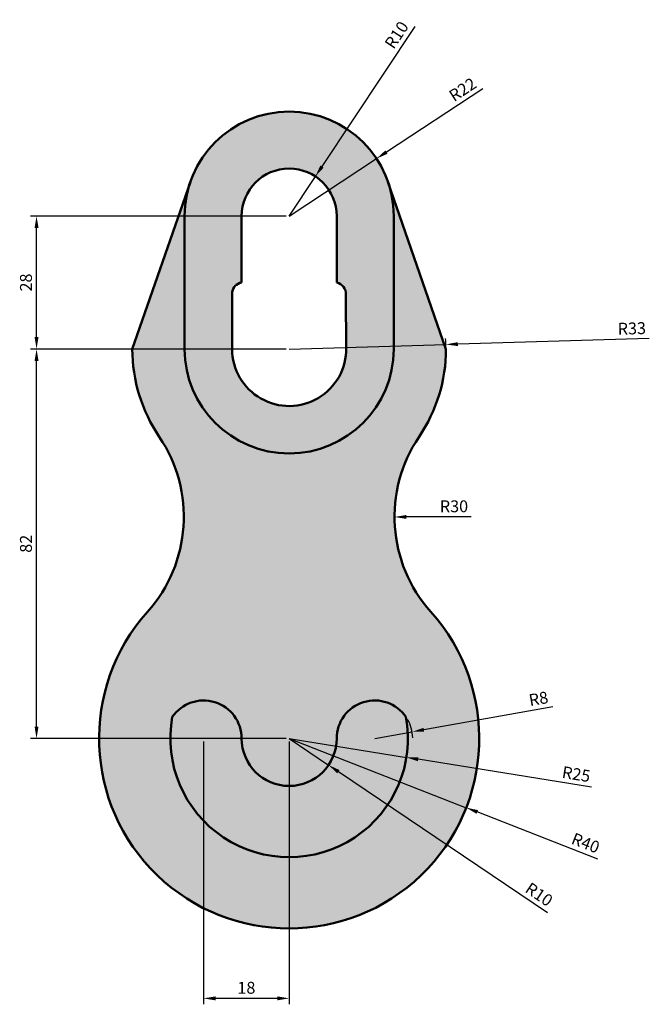
# Model space of a CAD drawing. Units: millimetres. Extents: x 3096 to 3229, y 1131 to 1338.
import ezdxf

# ---------------------------------------------------------------- set-up
doc = ezdxf.new("R2010")
doc.units = ezdxf.units.MM
for name, color, linetype, lineweight in [('M-DIMS', 2, 'Continuous', 25), ('M-HATC', 6, 'Continuous', 18), ('M-OUTL', 7, 'Continuous', 50)]:
    doc.layers.add(name, color=color, linetype=linetype, lineweight=lineweight)
doc.styles.get("Standard").update_dxf_attribs({"font": 'arial.ttf'})
doc.dimstyles.new('ISO-25', dxfattribs={"dimtxt": 2.5, "dimasz": 2.5, "dimexe": 1.25, "dimexo": 0.625, "dimtad": 1, "dimtxsty": 'Standard', "dimcen": 2.5, "dimadec": 0, "dimazin": 0, "dimtfac": 1, "dimtmove": 0, "dimatfit": 3, "dimfxl": 1, "dimarcsym": 0})

# ---------------------------------------------------------------- blocks, each defined once
blk = doc.blocks.new('*D1')
at = {"layer": 'Defpoints', "color": 0, "transparency": 16777216}
for p in [(3171.52, 1308.89), (3153.14, 1296.8)]:
    blk.add_point(p, dxfattribs=at)
at = {"layer": 'M-DIMS', "color": 0, "lineweight": -2, "transparency": 16777216}
for p, q in [((3193.86, 1323.58), (3173.61, 1310.26)), ((3153.14, 1296.8), (3171.52, 1308.89))]:
    blk.add_line(p, q, dxfattribs=at)
at = {"layer": 'M-DIMS', "color": 0, "transparency": 16777216}
blk.add_solid([(3173.38, 1310.61), (3173.84, 1309.91), (3171.52, 1308.89)], dxfattribs=at)
at = {"layer": 'M-DIMS', "color": 0, "transparency": 16777216, "insert": (3189.82, 1323.17), "char_height": 2.5, "attachment_point": 5, "rotation": 33.3268}
blk.add_mtext('R22', dxfattribs=at)
blk = doc.blocks.new('*D2')
at = {"layer": 'Defpoints', "color": 0, "transparency": 16777216}
for p in [(3158.66, 1305.14), (3153.14, 1296.8)]:
    blk.add_point(p, dxfattribs=at)
at = {"layer": 'M-DIMS', "color": 0, "lineweight": -2, "transparency": 16777216}
for p, q in [((3179.59, 1336.71), (3160.04, 1307.22)), ((3153.14, 1296.8), (3158.66, 1305.14))]:
    blk.add_line(p, q, dxfattribs=at)
at = {"layer": 'M-DIMS', "color": 0, "transparency": 16777216}
blk.add_solid([(3159.7, 1307.45), (3160.39, 1306.99), (3158.66, 1305.14)], dxfattribs=at)
at = {"layer": 'M-DIMS', "color": 0, "transparency": 16777216, "insert": (3176.01, 1334.75), "char_height": 2.5, "attachment_point": 5, "rotation": 56.4616}
blk.add_mtext('R10', dxfattribs=at)
blk = doc.blocks.new('*D3')
at = {"layer": 'Defpoints', "color": 0, "transparency": 16777216}
for p in [(3153.14, 1268.8), (3186.12, 1269.76)]:
    blk.add_point(p, dxfattribs=at)
at = {"layer": 'M-DIMS', "color": 0, "lineweight": -2, "transparency": 16777216}
for p, q in [((3228.92, 1271.01), (3188.62, 1269.84)), ((3153.14, 1268.8), (3186.12, 1269.76))]:
    blk.add_line(p, q, dxfattribs=at)
blk.add_arc((3153.14, 1268.8), 33, 1.0851, 3.843, dxfattribs=at)
at = {"layer": 'M-DIMS', "color": 0, "transparency": 16777216}
blk.add_solid([(3188.61, 1270.25), (3188.64, 1269.42), (3186.12, 1269.76)], dxfattribs=at)
at = {"layer": 'M-DIMS', "color": 0, "transparency": 16777216, "insert": (3225.25, 1272.81), "char_height": 2.5, "attachment_point": 5, "rotation": 1.6728}
blk.add_mtext('R33', dxfattribs=at)
blk = doc.blocks.new('*D4')
at = {"layer": 'Defpoints', "color": 0, "transparency": 16777216}
for p in [(3175.3, 1233.44), (3205.3, 1233.48)]:
    blk.add_point(p, dxfattribs=at)
at = {"layer": 'M-DIMS', "color": 0, "lineweight": -2, "transparency": 16777216}
blk.add_line((3191.43, 1233.46), (3177.8, 1233.45), dxfattribs=at)
at = {"layer": 'M-DIMS', "color": 0, "transparency": 16777216}
blk.add_solid([(3177.8, 1233.86), (3177.8, 1233.03), (3175.3, 1233.44)], dxfattribs=at)
at = {"layer": 'M-DIMS', "color": 0, "transparency": 16777216, "insert": (3187.82, 1235.36), "char_height": 2.5, "attachment_point": 5, "rotation": 0.0644}
blk.add_mtext('R30', dxfattribs=at)
blk = doc.blocks.new('*D5')
at = {"layer": 'Defpoints', "color": 0, "transparency": 16777216}
for p in [(3179.02, 1188.2), (3171.14, 1186.8)]:
    blk.add_point(p, dxfattribs=at)
at = {"layer": 'M-DIMS', "color": 0, "lineweight": -2, "transparency": 16777216}
for p, q in [((3208.6, 1193.44), (3181.48, 1188.63)), ((3171.14, 1186.8), (3179.02, 1188.2))]:
    blk.add_line(p, q, dxfattribs=at)
blk.add_arc((3171.14, 1186.8), 8, 1.1021, 30.1459, dxfattribs=at)
at = {"layer": 'M-DIMS', "color": 0, "transparency": 16777216}
blk.add_solid([(3181.4, 1189.04), (3181.55, 1188.22), (3179.02, 1188.2)], dxfattribs=at)
at = {"layer": 'M-DIMS', "color": 0, "transparency": 16777216, "insert": (3205.66, 1194.85), "char_height": 2.5, "attachment_point": 5, "rotation": 10.0546}
blk.add_mtext('R8', dxfattribs=at)
blk = doc.blocks.new('*D6')
at = {"layer": 'Defpoints', "color": 0, "transparency": 16777216}
for p in [(3153.14, 1186.8), (3177.82, 1182.81)]:
    blk.add_point(p, dxfattribs=at)
at = {"layer": 'M-DIMS', "color": 0, "lineweight": -2, "transparency": 16777216}
for p, q in [((3153.14, 1186.8), (3177.82, 1182.81)), ((3216.76, 1176.52), (3180.29, 1182.41))]:
    blk.add_line(p, q, dxfattribs=at)
at = {"layer": 'M-DIMS', "color": 0, "transparency": 16777216}
blk.add_solid([(3180.35, 1182.82), (3180.22, 1182), (3177.82, 1182.81)], dxfattribs=at)
at = {"layer": 'M-DIMS', "color": 0, "transparency": 16777216, "insert": (3213.49, 1178.97), "char_height": 2.5, "attachment_point": 5, "rotation": 350.8174}
blk.add_mtext('R25', dxfattribs=at)
blk = doc.blocks.new('*D7')
at = {"layer": 'Defpoints', "color": 0, "transparency": 16777216}
for p in [(3153.14, 1186.8), (3161.43, 1181.2)]:
    blk.add_point(p, dxfattribs=at)
at = {"layer": 'M-DIMS', "color": 0, "lineweight": -2, "transparency": 16777216}
for p, q in [((3153.14, 1186.8), (3161.43, 1181.2)), ((3207.47, 1150.11), (3163.5, 1179.8))]:
    blk.add_line(p, q, dxfattribs=at)
at = {"layer": 'M-DIMS', "color": 0, "transparency": 16777216}
blk.add_solid([(3163.73, 1180.15), (3163.26, 1179.46), (3161.43, 1181.2)], dxfattribs=at)
at = {"layer": 'M-DIMS', "color": 0, "transparency": 16777216, "insert": (3205.55, 1153.7), "char_height": 2.5, "attachment_point": 5, "rotation": 325.9669}
blk.add_mtext('R10', dxfattribs=at)
blk = doc.blocks.new('*D8')
at = {"layer": 'Defpoints', "color": 0, "transparency": 16777216}
for p in [(3153.14, 1186.8), (3190.39, 1172.23)]:
    blk.add_point(p, dxfattribs=at)
at = {"layer": 'M-DIMS', "color": 0, "lineweight": -2, "transparency": 16777216}
for p, q in [((3153.14, 1186.8), (3190.39, 1172.23)), ((3218.06, 1161.4), (3192.72, 1171.32))]:
    blk.add_line(p, q, dxfattribs=at)
at = {"layer": 'M-DIMS', "color": 0, "transparency": 16777216}
blk.add_solid([(3192.87, 1171.71), (3192.57, 1170.93), (3190.39, 1172.23)], dxfattribs=at)
at = {"layer": 'M-DIMS', "color": 0, "transparency": 16777216, "insert": (3215.4, 1164.49), "char_height": 2.5, "attachment_point": 5, "rotation": 338.6363}
blk.add_mtext('R40', dxfattribs=at)
blk = doc.blocks.new('*D9')
at = {"layer": 'Defpoints', "color": 0, "transparency": 16777216}
for p in [(3099.98, 1268.8), (3153.14, 1268.8), (3153.14, 1186.8)]:
    blk.add_point(p, dxfattribs=at)
at = {"layer": 'M-DIMS', "color": 0, "lineweight": -2, "transparency": 16777216}
for p, q in [((3152.51, 1268.8), (3098.73, 1268.8)), ((3099.98, 1189.3), (3099.98, 1266.3)), ((3152.51, 1186.8), (3098.73, 1186.8))]:
    blk.add_line(p, q, dxfattribs=at)
at = {"layer": 'M-DIMS', "color": 0, "transparency": 16777216}
for points in [[(3099.57, 1266.3), (3100.4, 1266.3), (3099.98, 1268.8)], [(3099.57, 1189.3), (3100.4, 1189.3), (3099.98, 1186.8)]]:
    blk.add_solid(points, dxfattribs=at)
at = {"layer": 'M-DIMS', "color": 0, "transparency": 16777216, "insert": (3098.08, 1227.8), "char_height": 2.5, "attachment_point": 5, "rotation": 90}
blk.add_mtext('82', dxfattribs=at)
blk = doc.blocks.new('*D10')
at = {"layer": 'Defpoints', "color": 0, "transparency": 16777216}
for p in [(3099.98, 1296.8), (3153.14, 1296.8), (3153.14, 1268.8)]:
    blk.add_point(p, dxfattribs=at)
at = {"layer": 'M-DIMS', "color": 0, "lineweight": -2, "transparency": 16777216}
for p, q in [((3152.51, 1296.8), (3098.73, 1296.8)), ((3099.98, 1271.3), (3099.98, 1294.3)), ((3152.51, 1268.8), (3098.73, 1268.8))]:
    blk.add_line(p, q, dxfattribs=at)
at = {"layer": 'M-DIMS', "color": 0, "transparency": 16777216}
for points in [[(3099.57, 1294.3), (3100.4, 1294.3), (3099.98, 1296.8)], [(3099.57, 1271.3), (3100.4, 1271.3), (3099.98, 1268.8)]]:
    blk.add_solid(points, dxfattribs=at)
at = {"layer": 'M-DIMS', "color": 0, "transparency": 16777216, "insert": (3098.08, 1282.8), "char_height": 2.5, "attachment_point": 5, "rotation": 90}
blk.add_mtext('28', dxfattribs=at)
blk = doc.blocks.new('*D11')
at = {"layer": 'Defpoints', "color": 0, "transparency": 16777216}
for p in [(3135.14, 1186.8), (3153.14, 1186.8), (3135.14, 1132.08)]:
    blk.add_point(p, dxfattribs=at)
at = {"layer": 'M-DIMS', "color": 0, "lineweight": -2, "transparency": 16777216}
for p, q in [((3135.14, 1186.18), (3135.14, 1130.83)), ((3153.14, 1186.18), (3153.14, 1130.83)), ((3150.64, 1132.08), (3137.64, 1132.08))]:
    blk.add_line(p, q, dxfattribs=at)
at = {"layer": 'M-DIMS', "color": 0, "transparency": 16777216}
for points in [[(3137.64, 1132.49), (3137.64, 1131.66), (3135.14, 1132.08)], [(3150.64, 1132.49), (3150.64, 1131.66), (3153.14, 1132.08)]]:
    blk.add_solid(points, dxfattribs=at)
at = {"layer": 'M-DIMS', "color": 0, "transparency": 16777216, "insert": (3144.14, 1133.98), "char_height": 2.5, "attachment_point": 5}
blk.add_mtext('18', dxfattribs=at)

msp = doc.modelspace()

# ---------------------------------------------------------------- hatches: boundary and pattern name
at = {"layer": 'M-HATC'}
h = msp.add_hatch(color=256, dxfattribs=at)
h.dxf.hatch_style = 1
h.set_gradient(color1=(255, 0, 255), color2=(255, 0, 255), tint=1)
h.paths.add_polyline_path([(3131.138, 1296.801), (3131.138, 1268.801, 1), (3175.138, 1268.801), (3175.138, 1296.801, 1)])
h.paths.add_polyline_path([(3163.138, 1296.801), (3163.138, 1282.801, -0.3877258), (3165.028, 1280.221), (3165.136, 1269.032, -1.0096804), (3141.138, 1268.801), (3141.138, 1280.691, -0.344834), (3143.138, 1282.801), (3143.138, 1296.801, -1)], flags=16)
h.paths.add_polyline_path([(3143.138, 1186.801, 0.7357684), (3128.555, 1191.346, 1.2018426), (3177.721, 1191.346, 0.7357684), (3163.138, 1186.801, -1)])
h = msp.add_hatch(color=256, dxfattribs=at)
h.dxf.hatch_style = 1
h.set_gradient(color1=(0, 0, 255), color2=(255, 255, 0), tint=1)
h.paths.add_polyline_path([(3182.947, 1213.473, -0.34396), (3180.463, 1250.298, 0.1499114), (3186.138, 1268.801), (3173.923, 1304.011, -0.0836763), (3175.138, 1296.801), (3175.138, 1268.801, -1), (3131.138, 1268.801), (3131.138, 1296.801, -0.0836763), (3132.353, 1304.011), (3120.138, 1268.801, 0.1499114), (3125.813, 1250.298, -0.34396), (3123.329, 1213.473, 2.2366525)])
h.paths.add_polyline_path([(3143.138, 1186.801, 1), (3163.138, 1186.801, -0.7357684), (3177.721, 1191.346, -1.2018426), (3128.555, 1191.346, -0.7357684)], flags=16)

# ---------------------------------------------------------------- linework, layer by layer
at = {"layer": 'M-OUTL'}
for p, q in [((3120.138, 1268.801), (3132.353, 1304.011)), ((3186.138, 1268.801), (3173.923, 1304.011)), ((3131.138, 1296.801), (3131.138, 1268.801)), ((3143.138, 1296.801), (3143.138, 1282.801)), ((3163.138, 1296.801), (3163.138, 1282.801)), ((3175.138, 1296.801), (3175.138, 1268.801)), ((3141.138, 1268.801), (3141.138, 1280.691)), ((3165.138, 1268.801), (3165.028, 1280.221))]:
    msp.add_line(p, q, dxfattribs=at)
for centre, radius, start, end in [((3153.138, 1296.801), 22, 0, 180), ((3153.138, 1296.801), 10, 0, 180), ((3143.485, 1280.468), 2.358, 98.47395, 174.57769), ((3162.67, 1280.476), 2.372, 353.84729, 78.61768), ((3153.138, 1268.801), 33, 180, 214.1032), ((3153.138, 1268.801), 22, 180, 0), ((3153.138, 1268.801), 12, 180, 1.10394), ((3153.138, 1268.801), 33, 325.8968, 0), ((3100.972, 1233.477), 30, 318.17852, 34.1032), ((3205.304, 1233.477), 30, 145.8968, 221.82148), ((3153.138, 1186.801), 40, 138.17852, 41.82148), ((3135.138, 1186.801), 8, 0, 145.37784), ((3171.138, 1186.801), 8, 34.62216, 180), ((3153.138, 1186.801), 25, 169.52469, 10.47531), ((3153.138, 1186.801), 10, 180, 0)]:
    msp.add_arc(centre, radius, start, end, dxfattribs=at)

# ---------------------------------------------------------------- dimensions: what is measured, and where the dimension line sits
at = {"layer": 'M-DIMS'}
for center, mpoint, picture, middle in [((3153.138, 1296.801), (3158.663, 1305.136), '*D2', (3177.599, 1333.704)), ((3153.138, 1296.801), (3171.52, 1308.888), '*D1', (3190.851, 1321.599)), ((3153.138, 1268.801), (3186.124, 1269.764), '*D3', (3225.305, 1270.908)), ((3205.304, 1233.477), (3175.304, 1233.444), '*D4', (3187.822, 1233.458)), ((3171.138, 1186.801), (3179.015, 1188.197), '*D5', (3205.995, 1192.981)), ((3153.138, 1186.801), (3177.818, 1182.811), '*D6', (3213.189, 1177.093)), ((3153.138, 1186.801), (3161.425, 1181.204), '*D7', (3204.481, 1152.126)), ((3153.138, 1186.801), (3190.389, 1172.229), '*D8', (3214.704, 1162.718))]:
    dim = msp.add_radius_dim(center=center, mpoint=mpoint, dimstyle='ISO-25', override={"dimclrd": 0, "dimclre": 0, "dimclrt": 0}, dxfattribs=at)
    dim.commit()
    dim.dimension.update_dxf_attribs({"geometry": picture, "text_midpoint": middle, "dimtype": 164})
for base, p1, p2, picture, middle in [((3099.983, 1296.801), (3153.138, 1268.801), (3153.138, 1296.801), '*D10', (3098.081, 1282.801)), ((3099.983, 1268.801), (3153.138, 1186.801), (3153.138, 1268.801), '*D9', (3098.081, 1227.801))]:
    dim = msp.add_linear_dim(base=base, p1=p1, p2=p2, angle=90, dimstyle='ISO-25', override={"dimclrd": 0, "dimclre": 0, "dimclrt": 0}, dxfattribs=at)
    dim.commit()
    dim.dimension.update_dxf_attribs({"geometry": picture, "text_midpoint": middle})
dim = msp.add_linear_dim(base=(3135.138, 1132.077), p1=(3153.138, 1186.801), p2=(3135.138, 1186.801), dimstyle='ISO-25', override={"dimclrd": 0, "dimclre": 0, "dimclrt": 0}, dxfattribs=at)
dim.commit()
dim.dimension.update_dxf_attribs({"geometry": '*D11', "text_midpoint": (3144.138, 1133.979)})

doc.saveas('drawing.dxf')
